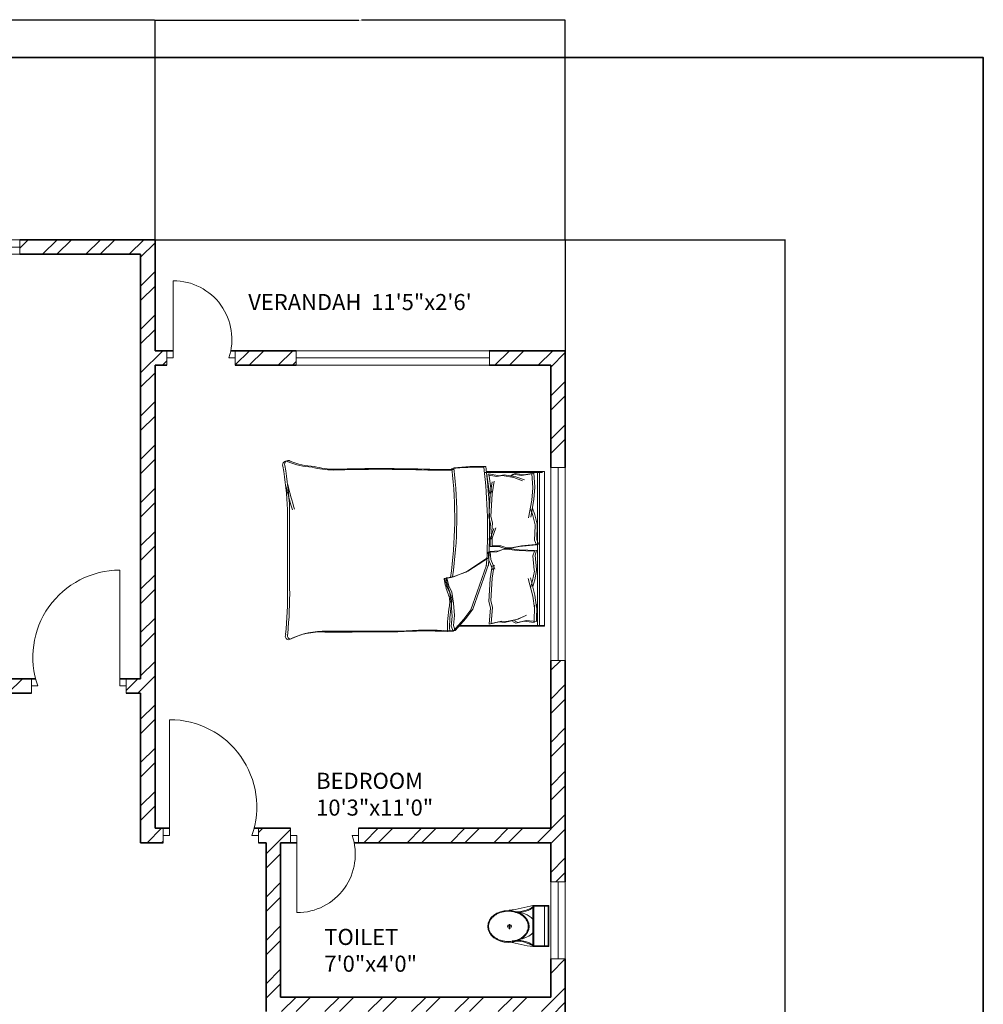
# Model space of a CAD drawing. Units: inches. Extents: x 1885 to 2748, y 783 to 2421.
# Tile 117 of 117: x 2449 to 2748, y 2115 to 2421. Entities that reach past the tile are written whole.
import ezdxf

# ---------------------------------------------------------------- set-up
doc = ezdxf.new("R2010")
doc.units = ezdxf.units.IN
for name, color, linetype, lineweight in [('A-ANNO-DIMS', 2, 'Continuous', 18), ('A-ANNO-TTLB', 7, 'Continuous', 35), ('A-AREA-IDEN', 7, 'Continuous', 18), ('A-DOOR', 31, 'Continuous', 18), ('A-FLOR-BALC', 7, 'Continuous', 25), ('A-FLOR-FIXT', 8, 'Continuous', 18), ('A-FURN', 8, 'Continuous', 13), ('A-GLAZ', 181, 'Continuous', 18), ('A-WALL', 7, 'Continuous', 35)]:
    doc.layers.add(name, color=color, linetype=linetype, lineweight=lineweight)
doc.layers.add('A-WALL-PATT', color=85, linetype='Continuous', lineweight=13, true_color=0x58ba48)
doc.styles.get("Standard").update_dxf_attribs({"font": 'arial.ttf'})
doc.dimstyles.get("Standard").update_dxf_attribs({"dimtxt": 0.18, "dimasz": 0.18, "dimexe": 0.18, "dimexo": 0.0625, "dimgap": 0.09, "dimtad": 0, "dimtih": 1, "dimtoh": 1, "dimdec": 4, "dimzin": 0, "dimdsep": 46, "dimtxsty": 'Standard', "dimcen": 0.09, "dimadec": 0, "dimazin": 0, "dimtfac": 1, "dimtdec": 4, "dimtofl": 0, "dimtmove": 0, "dimatfit": 3, "dimfxl": 1, "dimtolj": 1, "dimtzin": 0, "dimarcsym": 0})

# ---------------------------------------------------------------- blocks, each defined once
blk = doc.blocks.new('A$C31115884')
for p, q in [((283, 498), (223, 498)), ((258, 466), (258, 523)), ((0, 200), (0, 0)), ((520, 200), (0, 200)), ((10, 190), (10, 10)), ((510, 190), (10, 190)), ((510, 10), (510, 190)), ((520, 0), (520, 200)), ((510, 54), (0, 54)), ((10, 10), (510, 10)), ((0, 0), (520, 0))]:
    blk.add_line(p, q)
blk.add_circle((256, 496), 23.6)
for centre, radius, start, end in [((2778, -205), 2807, 165.4549, 171.7133), ((3237, 905), 2807, 188.2867, 194.5451), ((-295, 403), 365, 324.2091, 9.3499), ((-295, 403), 375, 324.2091, 9.3499), ((139, 406), 293, 315.8436, 2.6563), ((806, 403), 375, 179.2036, 215.7909), ((806, 403), 365, 170.6501, 215.7909), ((384, 406), 293, 190.2774, 224.1564)]:
    blk.add_arc(centre, radius, start, end)
blk.add_ellipse((256, 510), major_axis=(0, -261), ratio=0.772727)
blk.add_open_spline([(256, 259), (263, 259), (270, 260), (288, 262), (299, 265), (320, 273), (330, 278), (350, 291), (360, 299), (378, 316), (386, 326), (402, 347), (409, 358), (421, 383), (427, 395), (436, 422), (440, 436), (445, 465), (447, 480), (448, 509), (448, 524), (445, 553), (443, 568), (436, 596), (432, 610), (422, 636), (416, 649), (402, 672), (395, 683), (379, 703), (370, 712), (351, 728), (341, 735), (321, 746), (310, 751), (289, 757), (278, 759), (256, 761), (245, 761), (223, 757), (212, 754), (191, 746), (181, 741), (161, 728), (151, 720), (133, 703), (125, 693), (110, 672), (103, 660), (90, 636), (85, 623), (76, 596), (72, 582), (67, 553), (66, 538), (64, 509), (65, 494), (68, 465), (70, 450), (77, 422), (81, 408), (91, 382), (97, 370), (111, 346), (118, 335), (135, 316), (144, 307), (162, 291), (172, 284), (193, 273), (203, 269), (225, 262), (236, 260), (250, 259), (253, 259), (256, 259)], degree=3, knots=[0, 0, 0, 0, 0.110105, 0.110105, 0.285049, 0.285049, 0.459994, 0.459994, 0.634938, 0.634938, 0.809882, 0.809882, 0.984827, 0.984827, 1.159771, 1.159771, 1.334715, 1.334715, 1.50966, 1.50966, 1.684604, 1.684604, 1.859549, 1.859549, 2.034493, 2.034493, 2.209437, 2.209437, 2.384382, 2.384382, 2.559326, 2.559326, 2.73427, 2.73427, 2.909215, 2.909215, 3.084159, 3.084159, 3.259103, 3.259103, 3.434048, 3.434048, 3.608992, 3.608992, 3.783936, 3.783936, 3.958881, 3.958881, 4.133825, 4.133825, 4.30877, 4.30877, 4.483714, 4.483714, 4.658658, 4.658658, 4.833603, 4.833603, 5.008547, 5.008547, 5.183491, 5.183491, 5.358436, 5.358436, 5.53338, 5.53338, 5.708324, 5.708324, 5.883269, 5.883269, 6.058213, 6.058213, 6.233158, 6.233158, 6.283185, 6.283185, 6.283185, 6.283185])
blk = doc.blocks.new('BED-DOUBLE')
for p, q in [((27.75, 52.87), (24.5, 49.16)), ((27.75, 52.87), (24.5, 49.16)), ((28.39, 53.09), (25.14, 49.39)), ((28.39, 53.09), (25.14, 49.39)), ((29.49, 52.95), (27.75, 52.87, 3.87)), ((29.49, 52.95), (27.75, 52.87, 3.87)), ((28.37, 51.33), (27.75, 52.87)), ((28.37, 51.33), (27.75, 52.87)), ((30.13, 53.17), (28.39, 53.09, 3.87)), ((30.13, 53.17), (28.39, 53.09, 3.87)), ((29.01, 51.56), (28.39, 53.09)), ((29.01, 51.56), (28.39, 53.09)), ((0, 51.49), (0.64, 51.49)), ((0, 3.47), (0, 51.49)), ((0, 51.26), (26.61, 51.26)), ((0, 51.26), (26.61, 51.26)), ((0.64, 51.49), (27.25, 51.49)), ((0.64, 51.49), (27.25, 51.49)), ((1.54, 3.47), (1.54, 51.26)), ((1.54, 3.47), (1.54, 51.26)), ((2.18, 3.7), (2.18, 51.49)), ((2.18, 3.7), (2.18, 51.49)), ((2.56, 50.11), (2.46, 44.71)), ((2.56, 50.11), (2.46, 44.71)), ((2.56, 50.11), (5.77, 49.73)), ((2.56, 50.11), (5.77, 49.73)), ((3.2, 50.34), (3.1, 44.94)), ((3.2, 50.34), (3.1, 44.94)), ((3.2, 50.34), (6.41, 49.96)), ((3.2, 50.34), (6.41, 49.96)), ((8.26, 49.31), (5.58, 48.13)), ((8.26, 49.31), (5.58, 48.13)), ((5.77, 49.73), (8.34, 50.33)), ((5.77, 49.73), (8.34, 50.33)), ((8.9, 49.54), (6.22, 48.36)), ((8.9, 49.54), (6.22, 48.36)), ((6.41, 49.96), (8.98, 50.56)), ((6.41, 49.96), (8.98, 50.56)), ((11.83, 50.11), (8.26, 49.31)), ((11.83, 50.11), (8.26, 49.31)), ((8.34, 50.33), (9.39, 49.81)), ((8.34, 50.33), (9.39, 49.81)), ((12.47, 50.34), (8.9, 49.54)), ((12.47, 50.34), (8.9, 49.54)), ((8.98, 50.56), (10.03, 50.04)), ((8.98, 50.56), (10.03, 50.04)), ((13.44, 49.92), (11.83, 50.11)), ((13.44, 49.92), (11.83, 50.11)), ((14.08, 50.15), (12.47, 50.34)), ((14.08, 50.15), (12.47, 50.34)), ((16.58, 50.7), (13.44, 49.92)), ((16.58, 50.7), (13.44, 49.92)), ((17.22, 50.93), (14.08, 50.15)), ((17.22, 50.93), (14.08, 50.15)), ((16.17, 45.57), (16.58, 50.7)), ((16.17, 45.56), (16.58, 50.7)), ((16.81, 45.79), (17.22, 50.93)), ((16.81, 45.79), (17.22, 50.93)), ((24.5, 49.16), (22.33, 46.22)), ((24.5, 49.16), (22.33, 46.22)), ((25.14, 49.39), (22.97, 46.45)), ((25.14, 49.39), (22.97, 46.45)), ((28.06, 48.23), (28.37, 51.33)), ((28.06, 48.23), (28.37, 51.33)), ((28.7, 48.46), (29.01, 51.56)), ((28.7, 48.46), (29.01, 51.56)), ((3.1, 44.94), (3.19, 45.94)), ((3.1, 44.94), (3.19, 45.94)), ((3.19, 45.94), (3.71, 42.14)), ((3.19, 45.94), (3.71, 42.14)), ((22.33, 46.22), (20.32, 40.64)), ((22.33, 46.22), (20.32, 40.64)), ((22.97, 46.45), (20.96, 40.87)), ((22.97, 46.45), (20.96, 40.87)), ((28.37, 44.36), (28.06, 48.23)), ((28.37, 44.36), (28.06, 48.23)), ((29.01, 44.59), (28.7, 48.46)), ((29.01, 44.59), (28.7, 48.46)), ((2.46, 44.71), (2.55, 45.71)), ((2.46, 44.71), (2.55, 45.71)), ((2.55, 45.71), (3.07, 41.91)), ((2.55, 45.71), (3.07, 41.91)), ((16.73, 43.6), (16.17, 45.57)), ((16.73, 43.6), (16.17, 45.56)), ((16.3, 36.59), (16.73, 43.6)), ((16.3, 36.59), (16.73, 43.6)), ((17.37, 43.83), (16.81, 45.79)), ((17.37, 43.83), (16.81, 45.79)), ((16.94, 36.82), (17.37, 43.83)), ((16.94, 36.82), (17.37, 43.83)), ((28.83, 40.95), (28.37, 44.36)), ((28.83, 40.95), (28.37, 44.36)), ((29.47, 41.18), (29.01, 44.59)), ((29.47, 41.18), (29.01, 44.59)), ((3.07, 41.91), (4.43, 36.49)), ((3.07, 41.91), (4.43, 36.49)), ((3.71, 42.14), (5.07, 36.72)), ((3.71, 42.14), (5.07, 36.72)), ((20.32, 40.64), (17.39, 32.3)), ((20.32, 40.64), (17.39, 32.3)), ((20.96, 40.87), (18.03, 32.53)), ((20.96, 40.87), (18.03, 32.53)), ((29.76, 38.94), (28.83, 40.95)), ((29.76, 38.94), (28.83, 40.95)), ((30.4, 39.17), (29.47, 41.18)), ((30.4, 39.17), (29.47, 41.18)), ((79.89, 15.29), (79.89, 39.9)), ((79.89, 15.29), (79.89, 39.9)), ((3.08, 37.13), (2.54, 34.2)), ((3.08, 37.13), (2.54, 34.2)), ((3.68, 39.2), (3.08, 37.13)), ((3.68, 39.2), (3.08, 37.13)), ((3.72, 37.36), (3.18, 34.43)), ((3.72, 37.36), (3.18, 34.43)), ((4.32, 39.43), (3.72, 37.36)), ((4.32, 39.43), (3.72, 37.36)), ((16.27, 32.79), (16.94, 36.82)), ((16.27, 32.79), (16.94, 36.82)), ((30.38, 36.46), (29.76, 38.94)), ((30.38, 36.46), (29.76, 38.94)), ((31.02, 36.69), (30.4, 39.17)), ((31.02, 36.69), (30.4, 39.17)), ((79.25, 15.06), (79.25, 39.68)), ((79.25, 15.06), (79.25, 39.68)), ((2.54, 34.2), (2.56, 33.88)), ((2.54, 34.2), (2.56, 33.88)), ((2.56, 33.88), (2.98, 29.45)), ((2.56, 33.88), (2.98, 29.45)), ((3.18, 34.43), (3.2, 34.11)), ((3.18, 34.43), (3.2, 34.11)), ((3.2, 34.11), (3.62, 29.68)), ((3.2, 34.11), (3.62, 29.68)), ((16.74, 30.75), (15.46, 33.82)), ((16.74, 30.75), (15.46, 33.82)), ((15.63, 32.56), (16.3, 36.59)), ((15.63, 32.56), (16.3, 36.59)), ((17.38, 30.98), (16.1, 34.05)), ((17.38, 30.98), (16.1, 34.05)), ((17.39, 30.26), (23.88, 34.45)), ((17.39, 30.26), (23.88, 34.45)), ((18.03, 30.49), (24.52, 34.68)), ((18.03, 30.49), (24.52, 34.68)), ((23.88, 34.45), (28.37, 36.15)), ((23.88, 34.45), (28.37, 36.15)), ((24.52, 34.68), (29.01, 36.38)), ((24.52, 34.68), (29.01, 36.38)), ((28.37, 36.15), (30.38, 36.46)), ((28.37, 36.15), (30.38, 36.46)), ((29.01, 36.38), (31.02, 36.69)), ((29.01, 36.38), (31.02, 36.69)), ((16.9, 28.3), (16.74, 30.75)), ((16.9, 28.3), (16.74, 30.75)), ((17.54, 28.52), (17.38, 30.98)), ((17.54, 28.52), (17.38, 30.98)), ((2.98, 29.45), (2.5, 27.98)), ((2.98, 29.45), (2.5, 27.98)), ((2.5, 27.98), (7.87, 27.73)), ((2.5, 27.98), (7.87, 27.73)), ((3.62, 29.68), (3.13, 28.2)), ((3.62, 29.68), (3.13, 28.2)), ((3.13, 28.2), (8.51, 27.96)), ((3.13, 28.2), (8.51, 27.96)), ((7.87, 27.73), (11.08, 27.35)), ((7.87, 27.73), (11.08, 27.35)), ((8.51, 27.96), (11.72, 27.58)), ((8.51, 27.96), (11.72, 27.58)), ((11.72, 27.58), (13.02, 27.66)), ((11.72, 27.58), (13.02, 27.66)), ((12.38, 27.43), (14.22, 28.13)), ((12.38, 27.43), (14.22, 28.13)), ((13.02, 27.66), (14.86, 28.36)), ((13.02, 27.66), (14.86, 28.36)), ((14.22, 28.13), (16.9, 28.3)), ((14.22, 28.13), (16.9, 28.3)), ((14.86, 28.36), (17.54, 28.52)), ((14.86, 28.36), (17.54, 28.52)), ((1.87, 25.98), (7.22, 26.56)), ((1.87, 25.98), (7.22, 26.56)), ((2.45, 24.54), (1.87, 25.98)), ((2.45, 24.54), (1.87, 25.98)), ((2.31, 20.09), (2.45, 24.54)), ((2.31, 20.09), (2.45, 24.54)), ((2.51, 26.21), (7.86, 26.79)), ((2.51, 26.21), (7.86, 26.79)), ((3.09, 24.76), (2.51, 26.21)), ((3.09, 24.76), (2.51, 26.21)), ((2.95, 20.32), (3.09, 24.76)), ((2.95, 20.32), (3.09, 24.76)), ((7.22, 26.56), (10.4, 27.14)), ((7.22, 26.56), (10.4, 27.14)), ((7.86, 26.79), (11.04, 27.37)), ((7.86, 26.79), (11.04, 27.37)), ((10.4, 27.14), (11.71, 27.14)), ((10.4, 27.14), (11.71, 27.14)), ((11.04, 27.37), (12.35, 27.37)), ((11.04, 27.37), (12.35, 27.37)), ((11.08, 27.35), (12.38, 27.43)), ((11.08, 27.35), (12.38, 27.43)), ((11.71, 27.14), (13.59, 26.56)), ((11.71, 27.14), (13.59, 26.56)), ((12.35, 27.37), (14.22, 26.79)), ((12.35, 27.37), (14.22, 26.79)), ((13.59, 26.56), (16.27, 26.56)), ((13.59, 26.56), (16.27, 26.56)), ((14.22, 26.79), (16.91, 26.79)), ((14.22, 26.79), (16.91, 26.79)), ((16.17, 19.38), (16.58, 24.51)), ((16.17, 19.38), (16.58, 24.51)), ((16.27, 26.56), (16.27, 24.1)), ((16.27, 26.56), (16.27, 24.1)), ((16.81, 19.61), (17.22, 24.74)), ((16.81, 19.61), (17.22, 24.74)), ((16.91, 26.79), (16.91, 24.33)), ((16.91, 26.79), (16.91, 24.33)), ((16.27, 24.1), (15.18, 20.96)), ((16.27, 24.1), (15.18, 20.96)), ((16.91, 24.33), (15.82, 21.19)), ((16.91, 24.33), (15.82, 21.19)), ((2.31, 19.77), (2.31, 20.09)), ((2.31, 19.77), (2.31, 20.09)), ((3.03, 16.88), (2.31, 19.77)), ((3.03, 16.88), (2.31, 19.77)), ((2.95, 20), (2.95, 20.32)), ((2.95, 20), (2.95, 20.32)), ((3.67, 17.11), (2.95, 20)), ((3.67, 17.11), (2.95, 20)), ((16.73, 17.42), (16.17, 19.38)), ((16.73, 17.42), (16.17, 19.38)), ((17.37, 17.65), (16.81, 19.61)), ((17.37, 17.65), (16.81, 19.61)), ((3.75, 14.85), (3.03, 16.88)), ((3.75, 14.85), (3.03, 16.88)), ((3.32, 12.11), (4.33, 17.6)), ((3.32, 12.11), (4.33, 17.6)), ((4.39, 15.08), (3.67, 17.11)), ((4.39, 15.08), (3.67, 17.11)), ((3.96, 12.34), (4.97, 17.83)), ((3.96, 12.34), (4.97, 17.83)), ((16.3, 10.41), (16.73, 17.42)), ((16.3, 10.41), (16.73, 17.42)), ((16.94, 10.64), (17.37, 17.65)), ((16.94, 10.64), (17.37, 17.65)), ((3.67, 8.51), (3.96, 12.34)), ((3.67, 8.51), (3.96, 12.34)), ((3.03, 8.28), (3.32, 12.11)), ((3.03, 8.28), (3.32, 12.11)), ((15.63, 6.38), (16.3, 10.41)), ((15.63, 6.38), (16.3, 10.41)), ((16.27, 6.61), (16.94, 10.64)), ((16.27, 6.61), (16.94, 10.64)), ((16.3, 10.41), (16.62, 9.28)), ((16.3, 10.41), (16.62, 9.28)), ((16.62, 9.28), (17.34, 4.18)), ((16.62, 9.28), (17.34, 4.18)), ((16.94, 10.64), (17.26, 9.51)), ((16.94, 10.64), (17.26, 9.51)), ((17.26, 9.51), (17.98, 4.41)), ((17.26, 9.51), (17.98, 4.41)), ((3.01, 8.18), (3.03, 8.28)), ((3.01, 8.18), (3.03, 8.28)), ((3.34, 3.9), (3.01, 8.18)), ((3.34, 3.9), (3.01, 8.18)), ((3.65, 8.41), (3.67, 8.51)), ((3.65, 8.41), (3.67, 8.51)), ((3.98, 4.13), (3.65, 8.41)), ((3.98, 4.13), (3.65, 8.41)), ((9.6, 5.28), (6.85, 6.29)), ((9.6, 5.28), (6.85, 6.29)), ((18.11, 3.47), (0, 3.47)), ((18.11, 3.47), (0, 3.47)), ((18.75, 3.7), (0.64, 3.7)), ((18.75, 3.7), (0.64, 3.7)), ((3.32, 3.89), (6.5, 4.47)), ((3.32, 3.89), (6.5, 4.47)), ((3.96, 4.12), (7.14, 4.7)), ((3.96, 4.12), (7.14, 4.7)), ((8.96, 5.05), (6.21, 6.06)), ((8.96, 5.05), (6.21, 6.06)), ((6.5, 4.47), (9.1, 4.04)), ((6.5, 4.47), (9.1, 4.04)), ((7.14, 4.7), (9.74, 4.27)), ((7.14, 4.7), (9.74, 4.27)), ((12.57, 4.47), (8.96, 5.05)), ((12.57, 4.47), (8.96, 5.05)), ((9.1, 4.04), (10.12, 4.62)), ((9.1, 4.04), (10.12, 4.62)), ((13.21, 4.7), (9.6, 5.28)), ((13.21, 4.7), (9.6, 5.28)), ((9.74, 4.27), (10.75, 4.84)), ((9.74, 4.27), (10.75, 4.84)), ((14.16, 4.76), (12.57, 4.47)), ((14.16, 4.76), (12.57, 4.47)), ((14.8, 4.99), (13.21, 4.7)), ((14.8, 4.99), (13.21, 4.7)), ((17.34, 4.18), (14.16, 4.76)), ((17.34, 4.18), (14.16, 4.76)), ((17.98, 4.41), (14.8, 4.99)), ((17.98, 4.41), (14.8, 4.99))]:
    blk.add_line(p, q)
for centre, radius, start, end in [((68.67, 76.16), 23.07, 267.4714, 296.4681), ((68.67, 76.16), 23.07, 267.4714, 296.4681), ((69.31, 76.38), 23.07, 267.4714, 296.4681), ((69.31, 76.38), 23.07, 267.4714, 296.4681), ((78.87, 54.41), 1.1, 332.6588, 86.02), ((78.87, 54.41), 1.1, 332.6588, 86.02), ((79.51, 54.64), 1.1, 332.6588, 86.02), ((79.51, 54.64), 1.1, 332.6588, 86.02), ((-6.65, 51.33), 36.18, 349.8763, 2.5657), ((-6.65, 51.33), 36.18, 349.8763, 2.5657), ((36.32, 182.26), 129.5, 266.9791, 273.8365), ((36.32, 182.26), 129.5, 266.9791, 273.8365), ((-6.01, 51.55), 36.18, 349.8763, 2.5657), ((-6.01, 51.55), 36.18, 349.8763, 2.5657), ((36.96, 182.49), 129.5, 266.9791, 273.8365), ((36.96, 182.49), 129.5, 266.9791, 273.8365), ((67.83, -4508.74), 4561.86, 90.00217, 90.28689), ((67.83, -4508.75), 4561.86, 90.00217, 90.28689), ((68.46, -4508.52), 4561.86, 90.00217, 90.28689), ((68.46, -4508.52), 4561.86, 90.00217, 90.28689), ((212.28, 41.15), 133.04, 174.4998, 180.6351), ((212.28, 41.15), 133.04, 174.4998, 180.6351), ((212.92, 41.38), 133.04, 174.4998, 180.6351), ((212.92, 41.38), 133.04, 174.4998, 180.6351), ((35.07, 43.74), 6.22, 168.6608, 203.7384), ((35.07, 43.74), 6.22, 168.6608, 203.7384), ((35.71, 43.97), 6.22, 168.6608, 203.7384), ((35.71, 43.97), 6.22, 168.6608, 203.7384), ((1.49, 31.15), 29.65, 10.6617, 19.8806), ((1.49, 31.15), 29.65, 10.6617, 19.8806), ((2.13, 31.38), 29.65, 10.6617, 19.8806), ((2.13, 31.38), 29.65, 10.6617, 19.8806), ((31.08, 36.86), 0.185, 250.2464, 1.1377), ((31.08, 36.86), 0.185, 250.2464, 1.1377), ((156.32, 17.75), 129.02, 171.7845, 186.9006), ((156.32, 17.75), 129.02, 171.7845, 186.9006), ((156.96, 17.98), 129.02, 171.7845, 186.9006), ((156.96, 17.98), 129.02, 171.7845, 186.9006), ((30.44, 36.64), 0.185, 250.2464, 1.1377), ((30.44, 36.63), 0.185, 250.2464, 1.1377), ((182.06, 21.36), 164.97, 176.0865, 186.7821), ((182.06, 21.36), 164.97, 176.0865, 186.7821), ((182.7, 21.59), 164.97, 176.0865, 186.7821), ((182.7, 21.59), 164.97, 176.0865, 186.7821), ((-23.07, -16.99), 106.46, 13.3832, 17.7053), ((-23.07, -16.99), 106.46, 13.3832, 17.7053), ((-23.71, -17.22), 106.46, 13.3832, 17.7053), ((-23.71, -17.22), 106.46, 13.3832, 17.7053), ((200.84, 21.43), 121.76, 182.9958, 189.4091), ((200.84, 21.43), 121.76, 182.9958, 189.4091), ((201.48, 21.65), 121.76, 182.9958, 189.4091), ((201.48, 21.65), 121.76, 182.9958, 189.4091), ((20.1, 85.16), 83.31, 268.7218, 275.604), ((20.1, 85.16), 83.31, 268.7218, 275.604), ((20.74, 85.39), 83.31, 268.7218, 275.604), ((20.74, 85.39), 83.31, 268.7218, 275.604), ((31.18, -167.31), 170.11, 88.4762, 91.0082), ((31.18, -167.31), 170.11, 88.4762, 91.0082), ((31.82, -167.08), 170.11, 88.4762, 91.0082), ((31.82, -167.08), 170.11, 88.4762, 91.0082), ((50.62, 484.82), 482.31, 268.2277, 271.7185), ((50.62, 484.82), 482.31, 268.2277, 271.7185), ((51.26, 485.05), 482.31, 268.2277, 271.7185), ((51.26, 485.05), 482.31, 268.2277, 271.7185), ((64.52, -26.9), 29.63, 76.0648, 88.9113), ((64.52, -26.9), 29.63, 76.0648, 88.9113), ((65.16, -26.67), 29.63, 76.0648, 88.9113), ((65.16, -26.67), 29.63, 76.0648, 88.9113), ((70.28, -21.66), 23.56, 67.9751, 86.652), ((70.28, -21.66), 23.56, 67.9751, 86.652), ((70.92, -21.43), 23.56, 67.9751, 86.652), ((70.92, -21.43), 23.56, 67.9751, 86.652), ((79.72, 1.09), 1.09, 236.1736, 23.4781), ((79.72, 1.09), 1.09, 236.1736, 23.4781), ((80.36, 1.31), 1.09, 236.1736, 23.4781), ((80.36, 1.31), 1.09, 236.1736, 23.4781)]:
    blk.add_arc(centre, radius, start, end)
blk = doc.blocks.new('WIN-60')
for p, q in [((0, 60), (4.5, 60)), ((0, 60), (0, 0)), ((4.5, 60), (2.25, 60)), ((2.25, 60), (2.25, 0)), ((4.5, 0), (4.5, 60)), ((2.25, 0), (0, 0)), ((0, 0), (4.5, 0))]:
    blk.add_line(p, q)
blk = doc.blocks.new('WIN-24')
for p, q in [((0, 4.5), (0, 0)), ((0, 4.5), (24, 4.5)), ((24, 2.25), (24, 4.5)), ((24, 4.5), (24, 0)), ((0, 0), (0, 2.25)), ((0, 2.25), (24, 2.25)), ((24, 0), (0, 0))]:
    blk.add_line(p, q)
blk = doc.blocks.new('*D44')
at = {"layer": 'A-ANNO-DIMS', "color": 0, "lineweight": -2, "transparency": 16777216}
for p, q in [((2618.34, 2352.51), (2686.7, 2352.51)), ((2686.52, 2352.33), (2686.52, 1705.19)), ((2686.52, 1057.69), (2686.52, 1704.82)), ((2618.34, 1057.51), (2686.7, 1057.51))]:
    blk.add_line(p, q, dxfattribs=at)
at = {"layer": 'A-ANNO-DIMS', "color": 0, "transparency": 16777216}
for points in [[(2686.49, 2352.33), (2686.55, 2352.33), (2686.52, 2352.51)], [(2686.49, 1057.69), (2686.55, 1057.69), (2686.52, 1057.51)]]:
    blk.add_solid(points, dxfattribs=at)
at = {"layer": 'Defpoints', "color": 0, "transparency": 16777216}
for p in [(2618.27, 2352.51), (2686.52, 2352.51), (2618.27, 1057.51)]:
    blk.add_point(p, dxfattribs=at)
at = {"layer": 'A-ANNO-DIMS', "color": 0, "transparency": 16777216, "insert": (2686.52, 1705.01), "char_height": 0.18, "attachment_point": 5}
blk.add_mtext('\\A1;1295', dxfattribs=at)
blk = doc.blocks.new('*D53')
at = {"layer": 'A-ANNO-DIMS', "color": 0, "lineweight": -2, "transparency": 16777216}
for p, q in [((2358.77, 2352.57), (2358.77, 2420.94)), ((2358.95, 2420.76), (2424.49, 2420.76)), ((2490.59, 2420.76), (2425.05, 2420.76)), ((2490.77, 2352.57), (2490.77, 2420.94))]:
    blk.add_line(p, q, dxfattribs=at)
at = {"layer": 'A-ANNO-DIMS', "color": 0, "transparency": 16777216}
for points in [[(2358.95, 2420.79), (2358.95, 2420.73), (2358.77, 2420.76)], [(2490.59, 2420.79), (2490.59, 2420.73), (2490.77, 2420.76)]]:
    blk.add_solid(points, dxfattribs=at)
at = {"layer": 'Defpoints', "color": 0, "transparency": 16777216}
for p in [(2490.77, 2420.76), (2358.77, 2352.51), (2490.77, 2352.51)]:
    blk.add_point(p, dxfattribs=at)
at = {"layer": 'A-ANNO-DIMS', "color": 0, "transparency": 16777216, "insert": (2424.77, 2420.76), "char_height": 0.18, "attachment_point": 5}
blk.add_mtext('\\A1;132', dxfattribs=at)
blk = doc.blocks.new('*D54')
at = {"layer": 'A-ANNO-DIMS', "color": 0, "lineweight": -2, "transparency": 16777216}
for p, q in [((2490.77, 2352.57), (2490.77, 2420.94)), ((2490.95, 2420.76), (2554.14, 2420.76)), ((2618.09, 2420.76), (2554.91, 2420.76)), ((2618.27, 2352.57), (2618.27, 2420.94))]:
    blk.add_line(p, q, dxfattribs=at)
at = {"layer": 'A-ANNO-DIMS', "color": 0, "transparency": 16777216}
for points in [[(2490.95, 2420.79), (2490.95, 2420.73), (2490.77, 2420.76)], [(2618.09, 2420.79), (2618.09, 2420.73), (2618.27, 2420.76)]]:
    blk.add_solid(points, dxfattribs=at)
at = {"layer": 'Defpoints', "color": 0, "transparency": 16777216}
for p in [(2618.27, 2420.76), (2490.77, 2352.51), (2618.27, 2352.51)]:
    blk.add_point(p, dxfattribs=at)
at = {"layer": 'A-ANNO-DIMS', "color": 0, "transparency": 16777216, "insert": (2554.52, 2420.76), "char_height": 0.18, "attachment_point": 5}
blk.add_mtext('\\A1;127.5', dxfattribs=at)

msp = doc.modelspace()

# ---------------------------------------------------------------- hatches: boundary and pattern name
at = {"layer": 'A-WALL-PATT'}
h = msp.add_hatch(dxfattribs=at)
h.set_pattern_fill('ANSI32', color=256)
h.paths.add_polyline_path([(2007.77, 2318.01), (1980.77, 2318.01), (1980.77, 2281.22), (1985.27, 2281.22), (1985.27, 2313.51), (2007.77, 2313.51), (2007.77, 2315.76)])
h.paths.add_polyline_path([(2094.32, 2318.01), (2067.77, 2318.01), (2067.77, 2313.51), (2094.32, 2313.51), (2094.32, 2315.76)])
h.paths.add_polyline_path([(2131.37, 2315.76), (2131.37, 2318.01), (2131.19, 2318.01), (2112.61, 2318.01), (2112.61, 2313.51), (2117.27, 2313.51), (2117.27, 2255.2), (2121.77, 2255.2), (2121.77, 2313.51), (2131.37, 2313.51)])
h.paths.add_polyline_path([(2190.51, 2318.01), (2155.37, 2318.01), (2155.37, 2313.51), (2169.77, 2313.51), (2169.77, 2229.51), (2121.77, 2229.51), (2121.77, 2233.45), (2119.52, 2233.45), (2117.27, 2233.45), (2117.27, 2201.1), (2121.77, 2201.1), (2121.77, 2225.01), (2169.77, 2225.01), (2169.77, 2165.01), (2306.27, 2165.01), (2306.27, 2066.01), (2310.77, 2066.01), (2344.27, 2066.01), (2486.27, 2066.01), (2486.27, 1886.01), (2483.02, 1886.01), (2483.02, 1881.51), (2486.27, 1881.51), (2486.27, 1880.68), (2490.77, 1880.68), (2490.77, 2070.51), (2344.27, 2070.51), (2310.77, 2070.51), (2310.77, 2165.01), (2310.77, 2173.64), (2308.52, 2173.64), (2306.27, 2173.64), (2306.27, 2169.51), (2174.27, 2169.51), (2174.27, 2313.51), (2190.51, 2313.51), (2190.51, 2315.76)])
h.paths.add_polyline_path([(1985.27, 2221.22), (1980.77, 2221.22), (1980.77, 2165.01), (1992.77, 2165.01), (1992.77, 2141.93), (1997.27, 2141.93), (1997.27, 2165.01), (2117.27, 2165.01), (2117.27, 2163.13), (2121.77, 2163.13), (2121.77, 2172.73), (2119.52, 2172.73), (2117.27, 2172.73), (2117.27, 2169.51), (1985.27, 2169.51)])
h.paths.add_polyline_path([(1997.27, 2105.93), (1992.77, 2105.93), (1992.77, 2070.51), (2016.77, 2070.51), (2016.77, 2059.12), (2019.02, 2059.12), (2021.27, 2059.12), (2021.27, 2070.51), (2117.27, 2070.51), (2117.27, 2022.51), (2114.42, 2022.51), (2114.42, 2018.01), (2123.63, 2018.01), (2123.63, 2020.26), (2123.63, 2022.51), (2121.77, 2022.51), (2121.77, 2142.59), (2119.52, 2142.59), (2117.27, 2142.59), (2117.27, 2075.01), (1997.27, 2075.01)])
h.paths.add_polyline_path([(2092.03, 2020.26), (2092.03, 2022.51), (2021.27, 2022.51), (2021.27, 2035.12), (2016.77, 2035.12), (2016.77, 2018.01), (2016.77, 1978.78), (2021.27, 1978.78), (2021.27, 2018.01), (2092.03, 2018.01)])
h.paths.add_polyline_path([(2260.94, 2022.51), (2153.1, 2022.51), (2153.1, 2020.26), (2153.1, 2018.01), (2155.27, 2018.01), (2155.27, 1886.01), (2107.63, 1886.01), (2107.63, 1881.51), (2182.91, 1881.51), (2182.91, 1883.76), (2182.91, 1886.01), (2159.77, 1886.01), (2159.77, 2018.01), (2260.94, 2018.01), (2260.94, 2020.26)])
h.paths.add_polyline_path([(2047.63, 1883.76), (2047.63, 1886.01), (2021.27, 1886.01), (2021.27, 1918.78), (2019.02, 1918.78), (2016.77, 1918.78), (2016.77, 1881.51), (2047.63, 1881.51)])
h.paths.add_polyline_path([(2306.36, 1883.76), (2306.36, 1886.01), (2296.27, 1886.01), (2296.27, 1982.01), (2316.54, 1982.01), (2316.54, 1984.26), (2316.54, 1986.51), (2296.27, 1986.51), (2296.27, 2022.51), (2289.28, 2022.51), (2289.28, 2018.01), (2291.77, 2018.01), (2291.77, 1886.01), (2242.91, 1886.01), (2242.91, 1881.51), (2306.36, 1881.51)], flags=17)
h.paths.add_polyline_path([(1985.27, 1843.01), (2021.6, 1843.01), (2021.53, 1845.44), (2021.48, 1847.51), (1980.77, 1847.51), (1980.77, 1809.45), (1985.27, 1809.45)])
h.paths.add_polyline_path([(2131.48, 1845.26), (2131.48, 1847.51), (2081.53, 1847.51), (2081.53, 1843.01), (2117.27, 1843.01), (2117.27, 1784.15), (2119.52, 1784.15), (2121.77, 1784.15), (2121.77, 1843.01), (2131.48, 1843.01)])
h.paths.add_polyline_path([(2203.89, 1847.51), (2155.48, 1847.51), (2155.48, 1843.01), (2169.77, 1843.01), (2169.77, 1759.01), (2121.77, 1759.01), (2121.77, 1761.46), (2117.27, 1761.46), (2117.27, 1730.43), (2121.77, 1730.43), (2121.77, 1754.51), (2177.42, 1754.51), (2177.42, 1756.76), (2177.42, 1759.01), (2174.27, 1759.01), (2174.27, 1843.01), (2203.89, 1843.01)])
h.paths.add_polyline_path([(2335.55, 1845.26), (2335.55, 1847.51), (2239.89, 1847.51), (2239.89, 1843.01), (2306.27, 1843.01), (2306.27, 1759.01), (2199.49, 1759.01), (2199.49, 1754.51), (2310.77, 1754.51), (2310.77, 1843.01), (2335.55, 1843.01)])
h.paths.add_polyline_path([(2348.77, 2022.51), (2344.27, 2022.51), (2344.27, 1986.51), (2341.68, 1986.51), (2341.68, 1982.01), (2344.27, 1982.01), (2344.27, 1886.01), (2330.36, 1886.01), (2330.36, 1881.51), (2361.63, 1881.51), (2361.63, 1883.76), (2361.63, 1886.01), (2348.77, 1886.01)], flags=17)
h.paths.add_polyline_path([(2283.25, 2315.76), (2283.25, 2318.01), (2238.51, 2318.01), (2238.51, 2313.51), (2283.25, 2313.51)], flags=17)
h.paths.add_polyline_path([(2363.27, 2348.01), (2388.68, 2348.01), (2388.68, 2350.26), (2388.68, 2352.51), (2358.77, 2352.51), (2358.77, 2348.01), (2358.77, 2318.01), (2344.48, 2318.01), (2344.48, 2313.51), (2358.77, 2313.51), (2358.77, 2229.51), (2310.77, 2229.51), (2310.77, 2231.95), (2306.27, 2231.95), (2306.27, 2205.61), (2310.77, 2205.61), (2310.77, 2225.01), (2358.77, 2225.01), (2358.77, 2211.51), (2452.33, 2211.51), (2452.33, 2213.76), (2452.33, 2216.01), (2363.27, 2216.01), (2363.27, 2318.01)])
h.paths.add_polyline_path([(2310.77, 2313.51), (2320.48, 2313.51), (2320.48, 2315.76), (2320.48, 2318.01), (2302.73, 2318.01), (2302.73, 2313.51), (2306.27, 2313.51), (2306.27, 2251.08), (2310.77, 2251.08)], flags=17)
h.paths.add_polyline_path([(2490.77, 2352.51), (2486.27, 2352.51), (2448.68, 2352.51), (2448.68, 2348.01), (2486.27, 2348.01), (2486.27, 2318.01), (2486.27, 2216.01), (2481.78, 2216.01), (2481.78, 2211.51), (2486.27, 2211.51), (2486.27, 2165.01), (2493.29, 2165.01), (2493.29, 2167.26), (2493.29, 2169.51), (2490.77, 2169.51), (2490.77, 2313.51), (2494.43, 2313.51), (2494.43, 2318.01), (2490.77, 2318.01)])
h.paths.add_polyline_path([(2534.65, 2318.01), (2515.69, 2318.01), (2515.69, 2313.51), (2534.65, 2313.51), (2534.65, 2315.76)])
h.paths.add_polyline_path([(2618.27, 2318.01), (2594.65, 2318.01), (2594.65, 2313.51), (2613.77, 2313.51), (2613.77, 2281.71), (2618.27, 2281.71)])
h.paths.add_polyline_path([(2618.27, 2221.71), (2613.77, 2221.71), (2613.77, 2169.51), (2554.02, 2169.51), (2554.02, 2165.01), (2613.77, 2165.01), (2613.77, 2152.88), (2618.27, 2152.88)])
h.paths.add_polyline_path([(2618.27, 2128.88), (2616.02, 2128.88), (2613.77, 2128.88), (2613.77, 2117.01), (2529.77, 2117.01), (2529.77, 2165.01), (2532.85, 2165.01), (2532.85, 2169.51), (2522.87, 2169.51), (2522.87, 2165.01), (2525.27, 2165.01), (2525.27, 2117.01), (2525.27, 2112.51), (2525.27, 2108.58), (2529.77, 2108.58), (2529.77, 2112.51), (2613.77, 2112.51), (2613.77, 2080.19), (2618.27, 2080.19)])
h.paths.add_polyline_path([(2618.27, 2044.19), (2616.02, 2044.19), (2613.77, 2044.19), (2613.77, 2015.51), (2529.77, 2015.51), (2529.77, 2088.58), (2527.52, 2088.58), (2525.27, 2088.58), (2525.27, 2011.01), (2613.77, 2011.01), (2613.77, 1956.75), (2618.27, 1956.75)])
h.paths.add_polyline_path([(2618.27, 1881.51), (2618.27, 1896.75), (2613.77, 1896.75), (2613.77, 1881.51), (2613.77, 1847.51), (2592.71, 1847.51), (2592.71, 1843.01), (2613.77, 1843.01), (2613.77, 1765.01), (2613.77, 1760.51), (2609.62, 1760.51), (2609.62, 1756.01), (2613.77, 1756.01), (2613.77, 1660.01), (2608.54, 1660.01), (2608.54, 1655.51), (2613.77, 1655.51), (2613.77, 1508.16), (2618.27, 1508.16)])
h.paths.add_polyline_path([(2565.77, 1843.01), (2569, 1843.01), (2569, 1847.51), (2490.77, 1847.51), (2490.77, 1849.7), (2488.52, 1849.7), (2486.27, 1849.7), (2486.27, 1847.51), (2477.27, 1847.51), (2477.27, 1838.51), (2477.27, 1821.49), (2486.27, 1821.49), (2486.27, 1838.51), (2561.27, 1838.51), (2561.27, 1765.01), (2486.27, 1765.01), (2486.27, 1786.16), (2477.27, 1786.16), (2477.27, 1765.01), (2477.27, 1756.01), (2486.27, 1756.01), (2565.77, 1756.01), (2585.62, 1756.01), (2585.62, 1758.26), (2585.62, 1760.51), (2565.77, 1760.51), (2565.77, 1765.01)])
h.paths.add_polyline_path([(2486.27, 1651.01), (2561.27, 1651.01), (2561.27, 1567.01), (2486.27, 1567.01), (2486.27, 1591.32), (2477.27, 1591.32), (2477.27, 1567.01), (2477.27, 1558.01), (2477.27, 1555.44), (2481.77, 1555.44), (2481.77, 1558.01), (2568.65, 1558.01), (2568.65, 1560.26), (2568.65, 1562.51), (2565.77, 1562.51), (2565.77, 1655.51), (2584.54, 1655.51), (2584.54, 1657.76), (2584.54, 1660.01), (2565.77, 1660.01), (2486.27, 1660.01), (2477.27, 1660.01), (2477.27, 1651.01), (2477.27, 1632.99), (2486.27, 1632.99)])
h.paths.add_polyline_path([(2449.97, 1883.76), (2449.97, 1886.01), (2421.63, 1886.01), (2421.63, 1881.51), (2449.97, 1881.51)], flags=17)
h.paths.add_polyline_path([(2447.27, 1847.51), (2395.55, 1847.51), (2395.55, 1843.01), (2442.77, 1843.01), (2442.77, 1809.27), (2447.27, 1809.27)])
h.paths.add_polyline_path([(1985.27, 1749.45), (1980.77, 1749.45), (1980.77, 1694.5), (1985.27, 1694.5), (1985.27, 1694.51), (1986.9, 1694.51), (1986.9, 1697.78), (1986.9, 1699.01), (1985.27, 1699.01)])
h.paths.add_polyline_path([(2152.77, 1699.01), (2121.77, 1699.01), (2121.77, 1703.67), (2119.52, 1703.67), (2117.27, 1703.67), (2117.27, 1699.01), (2009.22, 1699.01), (2009.22, 1694.51), (2148.27, 1694.51), (2148.27, 1692.63), (2152.77, 1692.63)])
h.paths.add_polyline_path([(2016.27, 1694.51), (2011.77, 1694.51), (2011.77, 1558.01), (2040.81, 1558.01), (2040.81, 1560.26), (2040.81, 1562.51), (2016.27, 1562.51)])
h.paths.add_polyline_path([(2152.77, 1663.02), (2150.52, 1663.02), (2148.27, 1663.02), (2148.27, 1562.51), (2100.81, 1562.51), (2100.81, 1558.01), (2165.12, 1558.01), (2165.12, 1560.26), (2165.12, 1562.51), (2152.77, 1562.51), (2152.77, 1610.51), (2224.77, 1610.51), (2224.77, 1607.99), (2229.27, 1607.99), (2229.27, 1615.01), (2152.77, 1615.01)])
h.paths.add_polyline_path([(2238.61, 1560.26), (2238.61, 1562.51), (2229.27, 1562.51), (2229.27, 1588.76), (2227.02, 1588.76), (2224.77, 1588.77), (2224.77, 1562.51), (2189.12, 1562.51), (2189.12, 1558.01), (2238.61, 1558.01)])
h.paths.add_polyline_path([(2336.02, 1560.26), (2336.02, 1562.51), (2310.77, 1562.51), (2310.77, 1656.35), (2308.52, 1656.35), (2306.27, 1656.35), (2306.27, 1562.51), (2286.61, 1562.51), (2286.61, 1558.01), (2336.02, 1558.01)])
h.paths.add_polyline_path([(2447.27, 1690.97), (2445.02, 1690.97), (2442.77, 1690.97), (2442.77, 1687.01), (2306.27, 1687.01), (2306.27, 1680.75), (2310.77, 1680.75), (2310.77, 1682.51), (2442.77, 1682.51), (2442.77, 1562.51), (2396.02, 1562.51), (2396.02, 1558.01), (2447.27, 1558.01)])
h.paths.add_polyline_path([(2447.27, 1749.27), (2445.02, 1749.27), (2442.77, 1749.27), (2442.77, 1717.23), (2447.27, 1717.23)])
h.paths.add_polyline_path([(2044.67, 1521.76), (2044.67, 1524.01), (2007.27, 1524.01), (2007.27, 1503.49), (2009.52, 1503.49), (2011.77, 1503.49), (2011.77, 1519.51), (2044.67, 1519.51)])
h.paths.add_polyline_path([(2177.97, 1521.76), (2177.97, 1524.01), (2104.67, 1524.01), (2104.67, 1519.51), (2145.77, 1519.51), (2145.77, 1387.51), (2143.37, 1387.51), (2143.37, 1383.01), (2251.59, 1383.01), (2251.59, 1385.26), (2251.59, 1387.51), (2150.27, 1387.51), (2150.27, 1519.51), (2177.97, 1519.51)])
h.paths.add_polyline_path([(2298.7, 1524.01), (2237.97, 1524.01), (2237.97, 1519.51), (2282.27, 1519.51), (2282.27, 1387.51), (2279.68, 1387.51), (2279.68, 1383.01), (2286.77, 1383.01), (2286.77, 1419.01), (2312.45, 1419.01), (2312.45, 1421.26), (2312.45, 1423.51), (2286.77, 1423.51), (2286.77, 1519.51), (2298.7, 1519.51), (2298.7, 1521.72)], flags=17)
h.paths.add_polyline_path([(2361.9, 1521.76), (2361.9, 1524.01), (2322.7, 1524.01), (2322.7, 1519.51), (2334.77, 1519.51), (2334.77, 1423.51), (2331.93, 1423.51), (2331.93, 1419.01), (2334.77, 1419.01), (2334.77, 1387.51), (2334.77, 1383.23), (2339.27, 1383.23), (2339.27, 1387.51), (2339.27, 1519.51), (2361.9, 1519.51)], flags=17)
h.paths.add_polyline_path([(2447.27, 1521.76), (2447.27, 1524.01), (2421.9, 1524.01), (2421.9, 1519.51), (2447.27, 1519.51)], flags=17)
h.paths.add_polyline_path([(2481.77, 1529.6), (2479.52, 1529.6), (2477.27, 1529.6), (2477.27, 1524.01), (2474.49, 1524.01), (2474.49, 1519.51), (2477.27, 1519.51), (2477.27, 1334.51), (2296.77, 1334.51), (2296.77, 1240.51), (2160.27, 1240.51), (2160.27, 1180.51), (2112.27, 1180.51), (2112.27, 1207.69), (2110.02, 1207.69), (2107.77, 1207.69), (2107.77, 1171.61), (2112.27, 1171.61), (2112.27, 1176.01), (2160.27, 1176.01), (2160.27, 1092.01), (2144.22, 1092.01), (2144.22, 1087.51), (2189.5, 1087.51), (2189.5, 1089.76), (2189.5, 1092.01), (2164.77, 1092.01), (2164.77, 1236.01), (2296.77, 1236.01), (2296.77, 1231.91), (2301.27, 1231.91), (2301.27, 1330.01), (2481.77, 1330.01), (2481.77, 1387.51)])
h.paths.add_polyline_path([(2618.27, 1448.16), (2613.77, 1448.16), (2613.77, 1382.51), (2529.77, 1382.51), (2525.27, 1382.51), (2525.27, 1307.06), (2529.77, 1307.06), (2529.77, 1378.01), (2613.77, 1378.01), (2613.77, 1354.99), (2618.27, 1354.99)])
h.paths.add_polyline_path([(2618.27, 1318.99), (2613.77, 1318.99), (2613.77, 1281.01), (2529.77, 1281.01), (2529.77, 1283.79), (2527.52, 1283.79), (2525.27, 1283.79), (2525.27, 1228.51), (2516.79, 1228.51), (2516.79, 1224.01), (2533.48, 1224.01), (2533.48, 1226.26), (2533.48, 1228.51), (2529.77, 1228.51), (2529.77, 1276.51), (2613.77, 1276.51), (2613.77, 1266.02), (2618.27, 1266.02)])
h.paths.add_polyline_path([(2618.27, 1134.96), (2613.77, 1134.96), (2613.77, 1092.01), (2594.54, 1092.01), (2594.54, 1087.51), (2618.27, 1087.51)])
h.paths.add_polyline_path([(2534.54, 1092.01), (2509.77, 1092.01), (2509.77, 1087.51), (2534.54, 1087.51), (2534.54, 1089.76)])
h.paths.add_polyline_path([(2481.27, 1224.01), (2484.12, 1224.01), (2484.12, 1226.26), (2484.12, 1228.51), (2476.77, 1228.51), (2476.77, 1198.51), (2471.61, 1198.51), (2471.61, 1194.01), (2476.77, 1194.01), (2476.77, 1062.01), (2436.89, 1062.01), (2436.89, 1057.51), (2476.77, 1057.51), (2481.27, 1057.51), (2481.27, 1062.01), (2481.27, 1087.51), (2485.35, 1087.51), (2485.35, 1089.76), (2485.35, 1092.01), (2481.27, 1092.01), (2481.27, 1117.51)])
h.paths.add_polyline_path([(2439.9, 1198.51), (2349.27, 1198.51), (2349.27, 1194.01), (2349.27, 1180.51), (2301.27, 1180.51), (2301.27, 1201.9), (2299.02, 1201.9), (2296.77, 1201.9), (2296.77, 1172.34), (2299.02, 1172.34), (2301.27, 1172.34), (2301.27, 1176.01), (2349.27, 1176.01), (2349.27, 1092.01), (2334.45, 1092.01), (2334.45, 1087.51), (2349.27, 1087.51), (2349.27, 1057.51), (2353.77, 1057.51), (2376.89, 1057.51), (2376.89, 1059.76), (2376.89, 1062.01), (2353.77, 1062.01), (2353.77, 1087.51), (2353.77, 1180.51), (2353.77, 1194.01), (2439.9, 1194.01), (2439.9, 1196.26)])
h.paths.add_polyline_path([(2270.6, 1089.76), (2270.6, 1092.01), (2249.5, 1092.01), (2249.5, 1087.51), (2270.6, 1087.51)], flags=17)
h.paths.add_polyline_path([(2310.45, 1092.01), (2301.27, 1092.01), (2301.27, 1153.29), (2296.77, 1153.29), (2296.77, 1092.01), (2293.79, 1092.01), (2293.79, 1087.51), (2310.45, 1087.51), (2310.45, 1089.76)], flags=17)
h.paths.add_polyline_path([(2112.27, 1150.33), (2110.02, 1150.33), (2107.77, 1150.33), (2107.77, 1092.01), (2104.47, 1092.01), (2104.47, 1087.51), (2120.22, 1087.51), (2120.22, 1089.76), (2120.22, 1092.01), (2112.27, 1092.01)])
h.paths.add_polyline_path([(2082.17, 1092.01), (2058.14, 1092.01), (2058.14, 1087.51), (2082.17, 1087.51), (2082.17, 1089.76)])
h.paths.add_polyline_path([(1975.77, 1145.64), (1971.27, 1145.64), (1971.27, 1087.51), (1980.77, 1087.51), (1998.14, 1087.51), (1998.14, 1089.76), (1998.14, 1092.01), (1985.27, 1092.01), (1975.77, 1092.01)])
h.paths.add_polyline_path([(2112.27, 1244.38), (2110.02, 1244.38), (2107.77, 1244.38), (2107.77, 1240.51), (1992.27, 1240.51), (1992.27, 1271.01), (1987.77, 1271.01), (1987.77, 1240.51), (1980.77, 1240.51), (1975.77, 1240.51), (1971.27, 1240.51), (1971.27, 1205.64), (1975.77, 1205.64), (1975.77, 1236.01), (2107.77, 1236.01), (2107.77, 1233.44), (2112.27, 1233.44), (2112.27, 1236.01)])
h.paths.add_polyline_path([(2112.27, 1383.01), (2114.78, 1383.01), (2114.78, 1385.26), (2114.78, 1387.51), (2102.48, 1387.51), (2102.48, 1383.01), (2107.77, 1383.01), (2107.77, 1335.01), (2011.77, 1335.01), (2011.77, 1349.94), (2007.27, 1349.94), (2007.27, 1335.01), (1987.77, 1335.01), (1987.77, 1330.51), (1987.77, 1307.01), (1992.27, 1307.01), (1992.27, 1330.51), (2007.27, 1330.51), (2107.77, 1330.51), (2107.77, 1264.71), (2112.27, 1264.71)])
h.paths.add_polyline_path([(2077.86, 1387.51), (2011.77, 1387.51), (2011.77, 1390.04), (2009.52, 1390.04), (2007.27, 1390.04), (2007.27, 1373.94), (2011.77, 1373.94), (2011.77, 1383.01), (2077.86, 1383.01)])
h.paths.add_polyline_path([(2011.77, 1443.49), (2007.27, 1443.49), (2007.27, 1410.25), (2011.77, 1410.25)])

# ---------------------------------------------------------------- linework, layer by layer
at = {"layer": 'A-ANNO-TTLB'}
msp.add_lwpolyline([(1885.16, 2409.17), (2748.2, 2409.17), (2748.2, 922.58), (1885.16, 922.58)], close=True, dxfattribs=at)
at = {"layer": 'A-DOOR'}
for p, q in [((2496.43, 2315.76), (2496.43, 2339.76)), ((2494.43, 2318.01), (2494.43, 2313.51)), ((2494.43, 2313.51), (2494.43, 2318.01)), ((2515.69, 2318.01), (2515.69, 2313.51)), ((2494.43, 2315.76), (2496.43, 2315.76)), ((2515.69, 2315.76), (2513.69, 2315.76)), ((2515.69, 2313.51), (2515.69, 2315.76)), ((2479.78, 2213.76), (2479.78, 2249.76)), ((2452.33, 2216.01), (2452.33, 2211.51)), ((2452.33, 2211.51), (2452.33, 2213.76)), ((2452.33, 2213.76), (2454.33, 2213.76)), ((2481.78, 2213.76), (2479.78, 2213.76)), ((2481.78, 2216.01), (2481.78, 2211.51)), ((2481.78, 2211.51), (2481.78, 2213.76)), ((2495.29, 2167.26), (2495.29, 2203.26)), ((2493.29, 2169.51), (2493.29, 2165.01)), ((2522.87, 2169.51), (2522.87, 2165.01)), ((2532.85, 2165.01), (2532.85, 2169.51)), ((2532.85, 2169.51), (2532.85, 2167.26)), ((2554.02, 2169.51), (2554.02, 2165.01)), ((2493.29, 2165.01), (2493.29, 2167.26)), ((2493.29, 2167.26), (2495.29, 2167.26)), ((2522.87, 2167.26), (2520.87, 2167.26)), ((2522.87, 2165.01), (2522.87, 2167.26)), ((2532.85, 2167.26), (2534.85, 2167.26)), ((2534.85, 2167.26), (2534.85, 2143.26)), ((2554.02, 2167.26), (2552.02, 2167.26)), ((2554.02, 2165.01), (2554.02, 2167.26))]:
    msp.add_line(p, q, dxfattribs=at)
for centre, radius, start, end in [((2496.43, 2321.55), 18.21, 341.4517, 90), ((2479.78, 2222.76), 27, 90, 199.4824), ((2495.29, 2176.17), 27.09, 340.7878, 90), ((2534.85, 2161.4), 18.14, 270, 18.8338)]:
    msp.add_arc(centre, radius, start, end, dxfattribs=at)
at = {"layer": 'A-FLOR-BALC'}
for p, q in [((2490.77, 2352.51), (2618.27, 2352.51)), ((2618.27, 2352.51), (2618.27, 2318.01))]:
    msp.add_line(p, q, dxfattribs=at)
at = {"layer": 'A-WALL'}
for p, q in [((2448.68, 2352.51), (2486.27, 2352.51)), ((2486.27, 2352.51), (2490.77, 2352.51)), ((2490.77, 2352.51), (2490.77, 2318.01)), ((2448.68, 2348.01), (2486.27, 2348.01)), ((2486.27, 2348.01), (2486.27, 2318.01)), ((2486.27, 2318.01), (2486.27, 2216.01)), ((2490.77, 2318.01), (2496.43, 2318.01)), ((2514.29, 2318.01), (2534.65, 2318.01)), ((2594.65, 2318.01), (2618.27, 2318.01)), ((2618.27, 2318.01), (2618.27, 2281.71)), ((2490.77, 2313.51), (2490.77, 2169.51)), ((2490.77, 2313.51), (2494.43, 2313.51)), ((2515.69, 2313.51), (2534.65, 2313.51)), ((2594.65, 2313.51), (2613.77, 2313.51)), ((2613.77, 2313.51), (2613.77, 2281.71)), ((2613.77, 2221.71), (2613.77, 2169.51)), ((2618.27, 2221.71), (2618.27, 2152.88)), ((2363.27, 2216.01), (2453.64, 2216.01)), ((2479.78, 2216.01), (2486.27, 2216.01)), ((2358.77, 2211.51), (2452.33, 2211.51)), ((2481.78, 2211.51), (2486.27, 2211.51)), ((2486.27, 2211.51), (2486.27, 2165.01)), ((2490.77, 2169.51), (2495.29, 2169.51)), ((2521.54, 2169.51), (2532.85, 2169.51)), ((2529.77, 2169.51), (2525.27, 2169.51)), ((2554.02, 2169.51), (2613.77, 2169.51)), ((2486.27, 2165.01), (2493.29, 2165.01)), ((2522.87, 2165.01), (2525.27, 2165.01)), ((2525.27, 2165.01), (2525.27, 2117.01)), ((2529.77, 2117.01), (2529.77, 2165.01)), ((2529.77, 2165.01), (2534.85, 2165.01)), ((2552.63, 2165.01), (2613.77, 2165.01)), ((2613.77, 2165.01), (2613.77, 2152.88)), ((2613.77, 2165.01), (2613.77, 2152.88)), ((2613.77, 2128.88), (2613.77, 2117.01)), ((2613.77, 2128.88), (2613.77, 2117.01)), ((2618.27, 2128.88), (2618.27, 2080.19)), ((2525.27, 2117.01), (2525.27, 2112.51)), ((2613.77, 2117.01), (2529.77, 2117.01))]:
    msp.add_line(p, q, dxfattribs=at)

# ---------------------------------------------------------------- block references
at = {"layer": 'A-FLOR-FIXT', "xscale": 0.0246256636748975, "yscale": 0.0246256636748975, "zscale": 0.0246256636748975, "rotation": 90}
msp.add_blockref('A$C31115884', (2613.15, 2132.68), dxfattribs=at)
at = {"layer": 'A-FURN', "rotation": 180}
msp.add_blockref('BED-DOUBLE', (2611.84, 2283.86), dxfattribs=at)
at = {"layer": 'A-GLAZ', "extrusion": (0, 0, -1), "zscale": -1, "rotation": 90}
for p in [(-2388.68, 2348), (-2534.66, 2313.5)]:
    msp.add_blockref('WIN-60', p, dxfattribs=at)
at = {"layer": 'A-GLAZ'}
msp.add_blockref('WIN-60', (2613.77, 2221.71), dxfattribs=at)
at = {"layer": 'A-GLAZ', "rotation": 90}
msp.add_blockref('WIN-24', (2618.27, 2128.88), dxfattribs=at)

# ---------------------------------------------------------------- texts
at = {"layer": 'A-AREA-IDEN', "char_height": 5, "attachment_point": 1}
for s, width, insert in [('VERANDAH  11\'5"x2\'6\'', 98.5484, (2519.73, 2335.63)), ('BEDROOM\\P10\'3"x11\'0"', 124.3706, (2540.84, 2186.76)), ('TOILET\\P7\'0"x4\'0"', 96.2579, (2543.38, 2138.21))]:
    msp.add_mtext_dynamic_manual_height_columns(s, width=width, gutter_width=12.5, heights=[0], dxfattribs=dict(at, insert=insert))

# ---------------------------------------------------------------- dimensions: what is measured, and where the dimension line sits
at = {"layer": 'A-ANNO-DIMS'}
for base, p1, p2, override, picture, middle in [((2490.77, 2420.76), (2358.77, 2352.51), (2490.77, 2352.51), {"dimdec": 0, "dimlfac": 1, "dimrnd": 0, "dimzin": 0, "dimdsep": 46, "dimlunit": 2}, '*D53', (2424.77, 2420.76)), ((2618.27, 2420.76), (2490.77, 2352.51), (2618.27, 2352.51), {"dimdec": 1, "dimlfac": 1, "dimrnd": 0, "dimzin": 0, "dimdsep": 46, "dimlunit": 2}, '*D54', (2554.52, 2420.76))]:
    dim = msp.add_linear_dim(base=base, p1=p1, p2=p2, dimstyle='Standard', override=override, dxfattribs=at)
    dim.commit()
    dim.dimension.update_dxf_attribs({"geometry": picture, "text_midpoint": middle})
dim = msp.add_linear_dim(base=(2686.52, 2352.51), p1=(2618.27, 1057.51), p2=(2618.27, 2352.51), angle=90, dimstyle='Standard', override={"dimdec": 0, "dimlfac": 1, "dimrnd": 0, "dimzin": 0, "dimdsep": 46, "dimlunit": 2}, dxfattribs=at)
dim.commit()
dim.dimension.update_dxf_attribs({"geometry": '*D44', "text_midpoint": (2686.52, 1705.01)})

doc.saveas('drawing.dxf')
